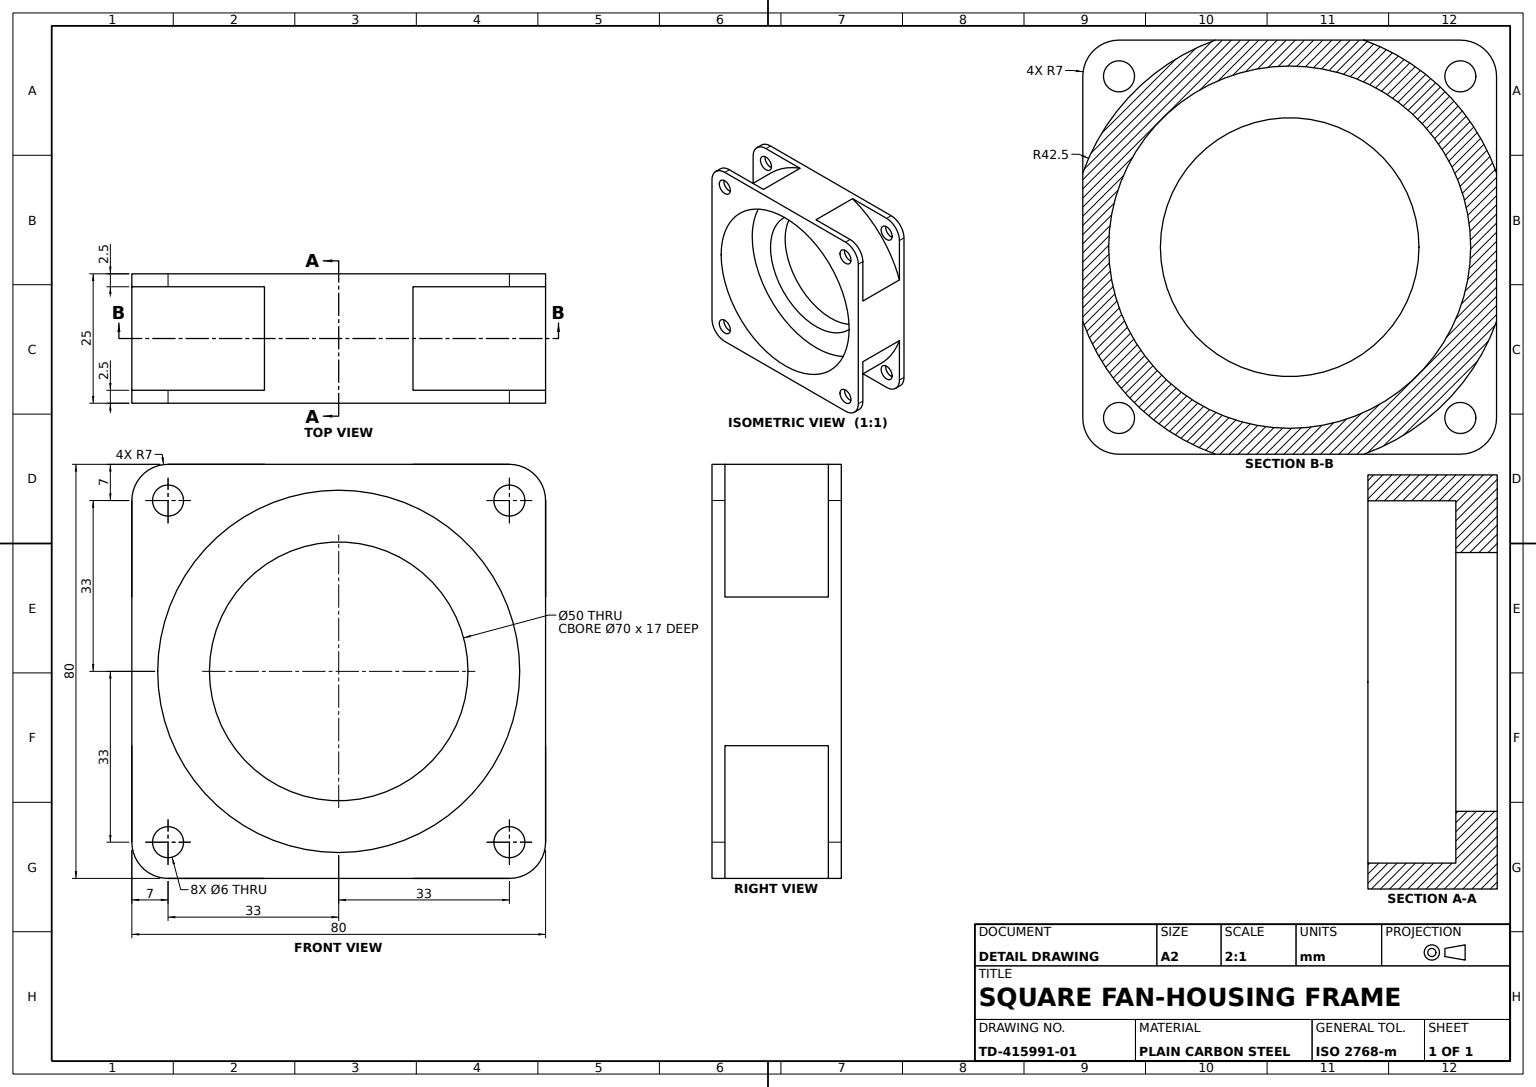
from build123d import *

# Parameters (mm, degrees)
FRONT_FLANGE_80X80_DEPTH = 2.5
HOUSING_BODY_DEPTH       = 20
REAR_FLANGE_80X80_DEPTH  = 2.5
MOUNTING_HOLES_SKETCH_R  = 3
MOUNTING_HOLES_4X_DEPTH  = 92.5
THROUGH_BORE_SKETCH_50_R = 25
THROUGH_BORE_50_DEPTH    = 132.5
COUNTERBORE_SKETCH_70_R  = 35
COUNTERBORE_70_DEPTH     = 17


with BuildPart() as part:
    # Front Flange Sketch → Front Flange 80x80 (new body)
    with BuildSketch(Plane.XY):
        with BuildLine():
            Line((-33, -40), (33, -40))
            ThreePointArc((33, -40), (37.949747468, -37.949747468), (40, -33))
            Line((40, -33), (40, 33))
            ThreePointArc((40, 33), (37.949747468, 37.949747468), (33, 40))
            Line((33, 40), (-33, 40))
            ThreePointArc((-33, 40), (-37.949747468, 37.949747468), (-40, 33))
            Line((-40, 33), (-40, -33))
            ThreePointArc((-40, -33), (-37.949747468, -37.949747468), (-33, -40))
        make_face()
    extrude(amount=-FRONT_FLANGE_80X80_DEPTH)

    # Housing Body Sketch → Housing Body (add)
    with BuildSketch(Plane(origin=(0, 0, -2.5), x_dir=(-1, 0, 0), z_dir=(0, 0, -1))):
        with BuildLine():
            Line((-14.361406616, 40), (14.361406616, 40))
            ThreePointArc((14.361406616, 40), (30.0520382, 30.0520382), (40, 14.361406616))
            Line((40, 14.361406616), (40, -14.361406616))
            ThreePointArc((40, -14.361406616), (30.0520382, -30.0520382), (14.361406616, -40))
            Line((14.361406616, -40), (-14.361406616, -40))
            ThreePointArc((-14.361406616, -40), (-30.0520382, -30.0520382), (-40, -14.361406616))
            Line((-40, -14.361406616), (-40, 14.361406616))
            ThreePointArc((-40, 14.361406616), (-30.0520382, 30.0520382), (-14.361406616, 40))
        make_face()
    extrude(amount=HOUSING_BODY_DEPTH)

    # Rear Flange Sketch → Rear Flange 80x80 (add)
    with BuildSketch(Plane(origin=(0, 0, -22.5), x_dir=(-1, 0, 0), z_dir=(0, 0, -1))):
        with BuildLine():
            Line((33, -40), (-33, -40))
            ThreePointArc((-33, -40), (-37.949747468, -37.949747468), (-40, -33))
            Line((-40, -33), (-40, 33))
            ThreePointArc((-40, 33), (-37.949747468, 37.949747468), (-33, 40))
            Line((-33, 40), (33, 40))
            ThreePointArc((33, 40), (37.949747468, 37.949747468), (40, 33))
            Line((40, 33), (40, -33))
            ThreePointArc((40, -33), (37.949747468, -37.949747468), (33, -40))
        make_face()
    extrude(amount=REAR_FLANGE_80X80_DEPTH)

    # Mounting Holes Sketch → Mounting Holes 4x (cut)
    with BuildSketch(Plane.XY):
        with Locations(Location((-33, 33, 0), (0, 0, 180))):
            Circle(MOUNTING_HOLES_SKETCH_R)
        with Locations(Location((33, 33, 0), (0, 0, 180))):
            Circle(MOUNTING_HOLES_SKETCH_R)
        with Locations(Location((33, -33, 0), (0, 0, 180))):
            Circle(MOUNTING_HOLES_SKETCH_R)
        with Locations(Location((-33, -33, 0), (0, 0, 180))):
            Circle(MOUNTING_HOLES_SKETCH_R)
    extrude(amount=-MOUNTING_HOLES_4X_DEPTH, mode=Mode.SUBTRACT)

    # Through Bore Sketch Ø50 → Through Bore Ø50 (cut)
    with BuildSketch(Plane.XY):
        Circle(THROUGH_BORE_SKETCH_50_R)
    extrude(amount=-THROUGH_BORE_50_DEPTH, mode=Mode.SUBTRACT)

    # Counterbore Sketch Ø70 → Counterbore Ø70 (cut)
    with BuildSketch(Plane.XY):
        Circle(COUNTERBORE_SKETCH_70_R)
    extrude(amount=-COUNTERBORE_70_DEPTH, mode=Mode.SUBTRACT)


solid = part.part
